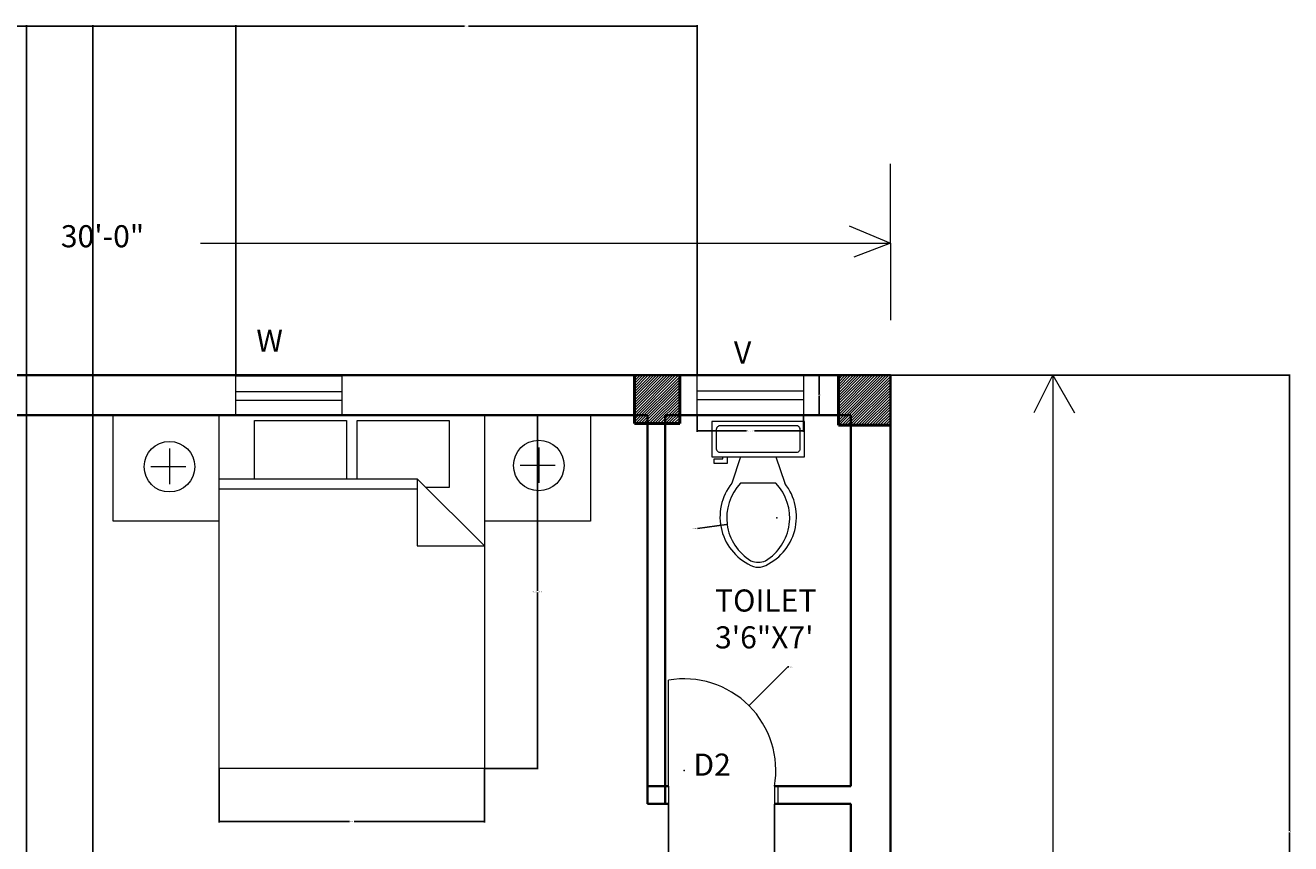
# Model space of a CAD drawing. Units: inches. Extents: x -12 to 472, y -585 to 99.
# Tile 4 of 4: x 186 to 472, y -86 to 99. Entities that reach past the tile are written whole.
import ezdxf

# ---------------------------------------------------------------- set-up
doc = ezdxf.new("R2010")
doc.units = ezdxf.units.IN
doc.header["$MEASUREMENT"] = 0
for name, color, linetype, lineweight in [('A-ANNO-DIMS', 2, 'Continuous', 18), ('A-ANNO-TEXT', 7, 'Continuous', 18), ('A-AREA-IDEN', 7, 'Continuous', 25), ('A-COLS', 7, 'Continuous', 50), ('A-COLS-PATT', 252, 'Continuous', 13), ('A-DOOR', 3, 'Continuous', 18), ('A-FLOR-FIXT', 9, 'Continuous', 20), ('A-FURN', 8, 'Continuous', 18), ('A-GLAZ', 4, 'Continuous', 18), ('A-WALL', 7, 'Continuous', 35)]:
    doc.layers.add(name, color=color, linetype=linetype, lineweight=lineweight)
doc.styles.get("Standard").update_dxf_attribs({"font": 'arial.ttf'})
doc.dimstyles.get("Standard").update_dxf_attribs({"dimtxt": 0.18, "dimasz": 0.18, "dimexe": 0.18, "dimexo": 0.0625, "dimgap": 0.09, "dimtad": 0, "dimtih": 1, "dimtoh": 1, "dimdec": 4, "dimzin": 0, "dimdsep": 46, "dimtxsty": 'Standard', "dimcen": 0.09, "dimadec": 0, "dimazin": 0, "dimtfac": 1, "dimtdec": 4, "dimtofl": 0, "dimtmove": 0, "dimatfit": 3, "dimfxl": 1, "dimtolj": 1, "dimtzin": 0, "dimarcsym": 0})
pattern_1 = [(45, (-1281.90016, -702.76037), (-0.30935922, 0.30935922), [])]

# ---------------------------------------------------------------- blocks, each defined once
blk = doc.blocks.new('Toilet - top')
for p, q in [((9.5, -6), (9.5, -2)), ((-10, -8.5), (-8, -8.5)), ((-10, -9.5), (-10, -8.5)), ((-8, -8.5), (-8, -8)), ((-7, -8), (-7, -9.5)), ((-4, -8), (-6, -14)), ((4, -8), (6, -14)), ((-7, -9.5), (-10, -9.5)), ((4, -14), (-4, -14))]:
    blk.add_line(p, q)
blk.add_lwpolyline([(10.5, -8), (10.5, 0), (-10.5, 0), (-10.5, -8)], close=True)
for points in [[(-9.5, -2), (-9.5, -6)], [(8.5, -1), (-8.5, -1)], [(-8.5, -7), (8.5, -7)]]:
    blk.add_lwpolyline(points)
for centre, radius, start, end in [((-8.62, -1.88), 0.884, 81.8699, 188.1301), ((8.62, -1.88), 0.884, 351.8699, 98.1301), ((-8.62, -6.12), 0.884, 171.8699, 278.1301), ((8.62, -6.12), 0.884, 261.8699, 8.1301), ((3.52, -21.58), 12.17, 141.4691, 247.9714), ((4.2, -21.82), 11.33, 136.3677, 238.9468), ((-3.52, -21.58), 12.17, 292.0284, 38.5307), ((-4.2, -21.82), 11.33, 301.053, 43.6321), ((0, -27.88), 4, 245.7318, 294.2682), ((0, -29), 4, 254.8605, 285.1395)]:
    blk.add_arc(centre, radius, start, end)
blk = doc.blocks.new('Bed - Queen')
for p, q in [((0, -80.00003), (0, 0)), ((0, 0), (59.99999, 0)), ((59.99999, 0), (59.99999, -80.00003)), ((7.99999, -1.2), (28.79998, -1.2)), ((7.99999, -14.4), (7.99999, -1.2)), ((28.79998, -1.2), (28.79998, -14.4)), ((31.19999, -1.2), (51.99999, -1.2)), ((31.19999, -14.4), (31.19999, -1.2)), ((51.99999, -1.2), (51.99999, -16.4)), ((0, -14.4), (44.8, -14.4)), ((44.8, -16.8), (0, -16.8)), ((59.99999, -29.6), (44.8, -14.4)), ((44.8, -14.4), (44.8, -29.6)), ((51.99999, -16.4), (46.79936, -16.4)), ((44.8, -29.6), (59.99999, -29.6)), ((59.99999, -80.00003), (0, -80.00003))]:
    blk.add_line(p, q)
blk = doc.blocks.new('WIN-24IN-EXT')
for p, q in [((0, 5.5), (24, 5.5)), ((0, 3.5), (24, 3.5))]:
    blk.add_line(p, q)
blk.add_lwpolyline([(0, 9), (24, 9), (24, 0), (0, 0)], close=True)
blk = doc.blocks.new('VENT-24IN-EXT')
for p, q in [((0, 5.5), (24, 5.5)), ((0, 3.5), (24, 3.5))]:
    blk.add_line(p, q)
blk.add_lwpolyline([(0, 9), (24, 9), (24, 0), (0, 0)], close=True)
blk = doc.blocks.new('NIGHTSTAND-24IN')
for p, q in [((0, 24), (24, 24)), ((24, 24), (24, 0)), ((24, 0), (0, 0))]:
    blk.add_line(p, q)
blk = doc.blocks.new('LAMP-BEDSIDE-PLAN')
for p, q in [((5.72, 9.81), (5.72, 1.79)), ((1.49, 5.8), (9.4, 5.8))]:
    blk.add_line(p, q)
blk.add_circle((5.72, 5.72), 5.72)
blk = doc.blocks.new('*D12')
at = {"layer": 'A-ANNO-DIMS', "color": 0, "lineweight": -2, "transparency": 16777216}
for p, q in [((337.57, 10.56), (337.57, 6.84)), ((361.57, 10.56), (361.57, 6.84)), ((337.75, 7.02), (348.67, 7.02)), ((361.39, 7.02), (350.48, 7.02))]:
    blk.add_line(p, q, dxfattribs=at)
at = {"layer": 'A-ANNO-DIMS', "color": 0, "transparency": 16777216}
for points in [[(337.75, 7.05), (337.75, 6.99), (337.57, 7.02)], [(361.39, 7.05), (361.39, 6.99), (361.57, 7.02)]]:
    blk.add_solid(points, dxfattribs=at)
at = {"layer": 'Defpoints', "color": 0, "transparency": 16777216}
for p in [(337.57, 10.62), (361.57, 10.62), (361.57, 7.02)]:
    blk.add_point(p, dxfattribs=at)
at = {"layer": 'A-ANNO-DIMS', "color": 0, "transparency": 16777216, "insert": (349.57, 7.02), "char_height": 0.18, "attachment_point": 5}
blk.add_mtext('\\A1;VENT 24 TYP.', dxfattribs=at)
blk = doc.blocks.new('*D13')
at = {"layer": 'A-ANNO-DIMS', "color": 0, "lineweight": -2, "transparency": 16777216}
for p, q in [((361.64, 19.62), (365.35, 19.62)), ((365.17, 19.44), (365.17, 15.3)), ((365.17, 10.8), (365.17, 14.94)), ((361.64, 10.62), (365.35, 10.62))]:
    blk.add_line(p, q, dxfattribs=at)
at = {"layer": 'A-ANNO-DIMS', "color": 0, "transparency": 16777216}
for points in [[(365.14, 19.44), (365.2, 19.44), (365.17, 19.62)], [(365.14, 10.8), (365.2, 10.8), (365.17, 10.62)]]:
    blk.add_solid(points, dxfattribs=at)
at = {"layer": 'Defpoints', "color": 0, "transparency": 16777216}
for p in [(361.57, 19.62), (365.17, 19.62), (361.57, 10.62)]:
    blk.add_point(p, dxfattribs=at)
at = {"layer": 'A-ANNO-DIMS', "color": 0, "transparency": 16777216, "insert": (365.17, 15.12), "char_height": 0.18, "attachment_point": 5}
blk.add_mtext('\\A1;9 TYP.', dxfattribs=at)
blk = doc.blocks.new('*D18')
at = {"layer": 'A-ANNO-DIMS', "color": 0, "lineweight": -2, "transparency": 16777216}
for p, q in [((289.49, 10.62), (301.61, 10.62)), ((301.43, 10.44), (301.43, -29.19)), ((301.43, -69.2), (301.43, -29.57)), ((289.49, -69.38), (301.61, -69.38))]:
    blk.add_line(p, q, dxfattribs=at)
at = {"layer": 'A-ANNO-DIMS', "color": 0, "transparency": 16777216}
for points in [[(301.4, 10.44), (301.46, 10.44), (301.43, 10.62)], [(301.4, -69.2), (301.46, -69.2), (301.43, -69.38)]]:
    blk.add_solid(points, dxfattribs=at)
at = {"layer": 'Defpoints', "color": 0, "transparency": 16777216}
for p in [(289.43, 10.62), (301.43, 10.62), (289.43, -69.38)]:
    blk.add_point(p, dxfattribs=at)
at = {"layer": 'A-ANNO-DIMS', "color": 0, "transparency": 16777216, "insert": (301.43, -29.38), "char_height": 0.18, "attachment_point": 5}
blk.add_mtext('\\A1;QUEEN BED 80 TYP.', dxfattribs=at)
blk = doc.blocks.new('*D19')
at = {"layer": 'A-ANNO-DIMS', "color": 0, "lineweight": -2, "transparency": 16777216}
for p, q in [((229.43, -69.44), (229.43, -81.56)), ((289.43, -69.44), (289.43, -81.56)), ((229.61, -81.38), (258.9, -81.38)), ((289.25, -81.38), (259.96, -81.38))]:
    blk.add_line(p, q, dxfattribs=at)
at = {"layer": 'A-ANNO-DIMS', "color": 0, "transparency": 16777216}
for points in [[(229.61, -81.35), (229.61, -81.41), (229.43, -81.38)], [(289.25, -81.35), (289.25, -81.41), (289.43, -81.38)]]:
    blk.add_solid(points, dxfattribs=at)
at = {"layer": 'Defpoints', "color": 0, "transparency": 16777216}
for p in [(229.43, -69.38), (289.43, -69.38), (289.43, -81.38)]:
    blk.add_point(p, dxfattribs=at)
at = {"layer": 'A-ANNO-DIMS', "color": 0, "transparency": 16777216, "insert": (259.43, -81.38), "char_height": 0.18, "attachment_point": 5}
blk.add_mtext('\\A1;60 TYP.', dxfattribs=at)
blk = doc.blocks.new('*D30')
at = {"layer": 'A-ANNO-DIMS', "color": 0, "lineweight": -2, "transparency": 16777216}
for p, q in [((185.8, -429.83), (185.8, 98.81)), ((185.98, 98.63), (193.09, 98.63)), ((200.62, 98.63), (193.51, 98.63)), ((200.8, -431.32), (200.8, 98.81))]:
    blk.add_line(p, q, dxfattribs=at)
at = {"layer": 'A-ANNO-DIMS', "color": 0, "transparency": 16777216}
for points in [[(185.98, 98.66), (185.98, 98.6), (185.8, 98.63)], [(200.62, 98.66), (200.62, 98.6), (200.8, 98.63)]]:
    blk.add_solid(points, dxfattribs=at)
at = {"layer": 'Defpoints', "color": 0, "transparency": 16777216}
for p in [(200.8, 98.63), (185.8, -429.9), (200.8, -431.38)]:
    blk.add_point(p, dxfattribs=at)
at = {"layer": 'A-ANNO-DIMS', "color": 0, "transparency": 16777216, "insert": (193.3, 98.63), "char_height": 0.18, "attachment_point": 5}
blk.add_mtext('\\A1;15', dxfattribs=at)
blk = doc.blocks.new('*D40')
at = {"layer": 'A-ANNO-DIMS', "color": 0, "lineweight": -2, "transparency": 16777216}
for p, q in [((331.04, -77.44), (331.04, -585.26)), ((355.04, -77.44), (355.04, -585.26)), ((331.22, -585.08), (342.82, -585.08)), ((354.86, -585.08), (343.26, -585.08))]:
    blk.add_line(p, q, dxfattribs=at)
at = {"layer": 'A-ANNO-DIMS', "color": 0, "transparency": 16777216}
for points in [[(331.22, -585.05), (331.22, -585.11), (331.04, -585.08)], [(354.86, -585.05), (354.86, -585.11), (355.04, -585.08)]]:
    blk.add_solid(points, dxfattribs=at)
at = {"layer": 'Defpoints', "color": 0, "transparency": 16777216}
for p in [(331.04, -77.38), (355.04, -77.38), (355.04, -585.08)]:
    blk.add_point(p, dxfattribs=at)
at = {"layer": 'A-ANNO-DIMS', "color": 0, "transparency": 16777216, "insert": (343.04, -585.08), "char_height": 0.18, "attachment_point": 5}
blk.add_mtext('\\A1;24', dxfattribs=at)
blk = doc.blocks.new('*D42')
at = {"layer": 'A-ANNO-DIMS', "color": 0, "lineweight": -2, "transparency": 16777216}
for p, q in [((74.01, 19.68), (74.01, 98.81)), ((74.19, 98.63), (153.13, 98.63)), ((232.97, 98.63), (154.04, 98.63)), ((233.15, 19.53), (233.15, 98.81))]:
    blk.add_line(p, q, dxfattribs=at)
at = {"layer": 'A-ANNO-DIMS', "color": 0, "transparency": 16777216}
for points in [[(74.19, 98.66), (74.19, 98.6), (74.01, 98.63)], [(232.97, 98.66), (232.97, 98.6), (233.15, 98.63)]]:
    blk.add_solid(points, dxfattribs=at)
at = {"layer": 'Defpoints', "color": 0, "transparency": 16777216}
for p in [(233.15, 98.63), (74.01, 19.62), (233.15, 19.47)]:
    blk.add_point(p, dxfattribs=at)
at = {"layer": 'A-ANNO-DIMS', "color": 0, "transparency": 16777216, "insert": (153.58, 98.63), "char_height": 0.18, "attachment_point": 5}
blk.add_mtext('\\A1;159.13', dxfattribs=at)
blk = doc.blocks.new('*D43')
at = {"layer": 'A-ANNO-DIMS', "color": 0, "lineweight": -2, "transparency": 16777216}
for p, q in [((233.15, 19.53), (233.15, 98.81)), ((233.33, 98.63), (284.91, 98.63)), ((337.39, 98.63), (285.81, 98.63)), ((337.57, 19.68), (337.57, 98.81))]:
    blk.add_line(p, q, dxfattribs=at)
at = {"layer": 'A-ANNO-DIMS', "color": 0, "transparency": 16777216}
for points in [[(233.33, 98.66), (233.33, 98.6), (233.15, 98.63)], [(337.39, 98.66), (337.39, 98.6), (337.57, 98.63)]]:
    blk.add_solid(points, dxfattribs=at)
at = {"layer": 'Defpoints', "color": 0, "transparency": 16777216}
for p in [(337.57, 98.63), (233.15, 19.47), (337.57, 19.62)]:
    blk.add_point(p, dxfattribs=at)
at = {"layer": 'A-ANNO-DIMS', "color": 0, "transparency": 16777216, "insert": (285.36, 98.63), "char_height": 0.18, "attachment_point": 5}
blk.add_mtext('\\A1;104.42', dxfattribs=at)
blk = doc.blocks.new('*D50')
at = {"layer": 'A-ANNO-DIMS', "color": 0, "lineweight": -2, "transparency": 16777216}
for p, q in [((381.34, 19.62), (471.69, 19.62)), ((471.51, 19.44), (471.51, -83.45)), ((471.51, -186.7), (471.51, -83.81)), ((381.34, -186.88), (471.69, -186.88))]:
    blk.add_line(p, q, dxfattribs=at)
at = {"layer": 'A-ANNO-DIMS', "color": 0, "transparency": 16777216}
for points in [[(471.48, 19.44), (471.54, 19.44), (471.51, 19.62)], [(471.48, -186.7), (471.54, -186.7), (471.51, -186.88)]]:
    blk.add_solid(points, dxfattribs=at)
at = {"layer": 'Defpoints', "color": 0, "transparency": 16777216}
for p in [(381.28, 19.62), (381.28, -186.88), (471.51, -186.88)]:
    blk.add_point(p, dxfattribs=at)
at = {"layer": 'A-ANNO-DIMS', "color": 0, "transparency": 16777216, "insert": (471.51, -83.63), "char_height": 0.18, "attachment_point": 5}
blk.add_mtext('\\A1;206.5', dxfattribs=at)
blk = doc.blocks.new('*D59')
at = {"layer": 'A-ANNO-DIMS', "color": 0, "lineweight": -2, "transparency": 16777216}
for p, q in [((358.07, -46.35), (349.4, -55.02)), ((358.25, -46.35), (358.07, -46.35)), ((334.51, -69.82), (334.69, -69.82)), ((334.6, -69.91), (334.6, -69.73))]:
    blk.add_line(p, q, dxfattribs=at)
at = {"layer": 'A-ANNO-DIMS', "color": 0, "transparency": 16777216}
blk.add_solid([(349.38, -55), (349.42, -55.04), (349.27, -55.15)], dxfattribs=at)
at = {"layer": 'Defpoints', "color": 0, "transparency": 16777216}
for p in [(349.27, -55.15), (334.6, -69.82)]:
    blk.add_point(p, dxfattribs=at)
at = {"layer": 'A-ANNO-DIMS', "color": 0, "transparency": 16777216, "insert": (358.81, -46.35), "char_height": 0.18, "attachment_point": 5}
blk.add_mtext('\\A1;R20.745', dxfattribs=at)
blk = doc.blocks.new('*D63')
at = {"layer": 'A-ANNO-DIMS', "color": 0, "lineweight": -2, "transparency": 16777216}
for p, q in [((337.59, -15.05), (344.15, -14.17)), ((355.47, -12.63), (355.65, -12.63)), ((355.56, -12.72), (355.56, -12.54))]:
    blk.add_line(p, q, dxfattribs=at)
at = {"layer": 'A-ANNO-DIMS', "color": 0, "transparency": 16777216}
blk.add_solid([(344.15, -14.14), (344.16, -14.2), (344.33, -14.15)], dxfattribs=at)
at = {"layer": 'Defpoints', "color": 0, "transparency": 16777216}
for p in [(344.33, -14.15), (355.56, -12.63)]:
    blk.add_point(p, dxfattribs=at)
at = {"layer": 'A-ANNO-DIMS', "color": 0, "transparency": 16777216, "insert": (336.92, -15.05), "char_height": 0.18, "attachment_point": 5}
blk.add_mtext('\\A1;4X R11.33', dxfattribs=at)

msp = doc.modelspace()

# ---------------------------------------------------------------- hatches: boundary and pattern name
at = {"layer": 'A-COLS-PATT'}
h = msp.add_hatch(dxfattribs=at)
h.set_pattern_fill('ANSI31', color=256, scale=3.5)
h.set_pattern_definition(pattern_1)
h.paths.add_polyline_path([(333.5896, 19.6212), (323.3586, 19.6212), (323.3586, 10.6212), (326.2783, 10.6212), (326.2783, 8.6749), (330.2783, 8.6749), (330.2783, 10.6212), (333.5896, 10.6212)])
h.paths.add_polyline_path([(326.2783, 10.6212), (323.3586, 10.6212), (323.3586, 8.6749), (326.2783, 8.6749)], flags=17)
h.paths.add_polyline_path([(333.5896, 10.6212), (330.2783, 10.6212), (330.2783, 8.6749), (333.5896, 8.6749)], flags=17)
h = msp.add_hatch(dxfattribs=at)
h.set_pattern_fill('ANSI31', color=256, scale=3.5)
h.set_pattern_definition(pattern_1)
h.paths.add_polyline_path([(381.2783, 19.6212), (369.4843, 19.6212), (369.4843, 10.6212), (372.2783, 10.6212), (372.2783, 8.3052), (381.2783, 8.3052)])
h.paths.add_polyline_path([(372.2783, 10.6212), (369.4843, 10.6212), (369.4843, 8.3052), (372.2783, 8.3052)], flags=17)

# ---------------------------------------------------------------- linework, layer by layer
at = {"layer": 'A-ANNO-DIMS'}
for p, q in [((381.2783, 49.4723), (381.2783, 67.4273)), ((371.9373, 53.4061), (381.2783, 49.4723)), ((225.2164, 49.4723), (381.2783, 49.4723)), ((381.2783, 49.4723), (373.0078, 46.3222)), ((381.2783, 49.4723), (381.2783, 32.0533)), ((395.6851, 19.6212), (440.3096, 19.6212)), ((413.8214, 11.17), (417.9974, 19.6212)), ((417.9974, 19.6212), (417.9974, -233.6801)), ((417.9974, 19.6212), (422.9031, 11.1243))]:
    msp.add_line(p, q, dxfattribs=at)
at = {"layer": 'A-COLS'}
for p, q in [((323.3586, 19.6212), (323.3586, 8.6749)), ((333.5896, 8.6749), (333.5896, 19.6212)), ((369.4843, 19.6212), (369.4843, 8.3052)), ((323.3586, 8.6749), (333.5896, 8.6749)), ((369.4843, 8.3052), (381.2783, 8.3052))]:
    msp.add_line(p, q, dxfattribs=at)
at = {"layer": 'A-DOOR'}
for p, q in [((331.0411, -73.3788), (331.0411, -49.3788)), ((331.0411, -73.3788), (331.0411, -77.3788)), ((355.0411, -73.3788), (355.0411, -77.3788)), ((355.8166, -73.3788), (355.8166, -77.3788))]:
    msp.add_line(p, q, dxfattribs=at)
msp.add_arc((334.6042, -69.8156), 20.7452, 350.10998, 99.89002, dxfattribs=at)
at = {"layer": 'A-WALL'}
for p, q in [((178.2783, 10.6212), (326.2783, 10.6212)), ((326.2783, 10.6212), (326.2783, -77.3788)), ((330.2783, 10.6212), (330.2783, -77.3788)), ((330.2783, 10.6212), (372.2783, 10.6212)), ((372.2783, 10.6212), (372.2783, -73.3788)), ((326.2783, -73.3788), (331.0411, -73.3788)), ((355.0411, -73.3788), (372.2783, -73.3788)), ((326.2783, -77.3788), (331.0411, -77.3788)), ((355.0411, -77.3788), (372.2783, -77.3788)), ((372.2783, -77.3788), (372.2783, -133.3788))]:
    msp.add_line(p, q, dxfattribs=at)
msp.add_lwpolyline([(21.2783, 19.6212), (381.2783, 19.6212), (381.2783, -526.3788), (21.2783, -526.3788)], close=True, dxfattribs=at)

# ---------------------------------------------------------------- block references
at = {"layer": 'A-FLOR-FIXT'}
msp.add_blockref('Toilet - top', (351.3581, 9.1824), dxfattribs=at)
at = {"layer": 'A-FURN', "rotation": 180}
msp.add_blockref('NIGHTSTAND-24IN', (229.428, 10.6214), dxfattribs=at)
at = {"layer": 'A-FURN'}
for name, p in [('Bed - Queen', (229.428, 10.6212)), ('NIGHTSTAND-24IN', (289.428, -13.3789)), ('LAMP-BEDSIDE-PLAN', (212.4458, -6.7945)), ('LAMP-BEDSIDE-PLAN', (295.9994, -6.5204))]:
    msp.add_blockref(name, p, dxfattribs=at)
at = {"layer": 'A-GLAZ'}
for name, p in [('WIN-24IN-EXT', (233.1479, 10.4678)), ('VENT-24IN-EXT', (337.573, 10.621))]:
    msp.add_blockref(name, p, dxfattribs=at)

# ---------------------------------------------------------------- texts
at = {"layer": 'A-ANNO-DIMS', "insert": (193.5858, 53.578), "char_height": 5, "attachment_point": 1}
msp.add_mtext_dynamic_manual_height_columns('30\'-0"', width=25.438653, gutter_width=25, heights=[0], dxfattribs=at)
at = {"layer": 'A-ANNO-TEXT', "char_height": 5, "attachment_point": 1}
for s, width, insert in [('W', 11.331186, (237.8264, 29.9341)), ('V', 17.014562, (345.8614, 27.2685)), ('D2', 15.456514, (336.686, -65.9853))]:
    msp.add_mtext_dynamic_manual_height_columns(s, width=width, gutter_width=25, heights=[0], dxfattribs=dict(at, insert=insert))
at = {"layer": 'A-AREA-IDEN', "insert": (341.5854, -28.8525), "char_height": 5, "attachment_point": 1}
msp.add_mtext_dynamic_manual_height_columns('TOILET\\P3\'6"X7\'', width=38.514755, gutter_width=25, heights=[0], dxfattribs=at)

# ---------------------------------------------------------------- dimensions: what is measured, and where the dimension line sits
at = {"layer": 'A-ANNO-DIMS'}
for base, p1, p2, override, picture, middle in [((233.1482, 98.6273), (74.0143, 19.6212), (233.1482, 19.468), {"dimdec": 2, "dimlfac": 1, "dimrnd": 0, "dimzin": 0, "dimdsep": 46, "dimlunit": 2}, '*D42', (153.5813, 98.6273)), ((200.803, 98.6273), (185.8034, -429.897), (200.803, -431.3788), {"dimdec": 0, "dimlfac": 1, "dimrnd": 0, "dimzin": 0, "dimdsep": 46, "dimlunit": 2}, '*D30', (193.3032, 98.6273)), ((337.5728, 98.6273), (233.1482, 19.468), (337.5728, 19.6212), {"dimdec": 2, "dimlfac": 1, "dimrnd": 0, "dimzin": 0, "dimdsep": 46, "dimlunit": 2}, '*D43', (285.3605, 98.6273)), ((355.0411, -585.0813), (331.0411, -77.3788), (355.0411, -77.3788), {"dimdec": 0, "dimlfac": 1, "dimrnd": 0, "dimzin": 0, "dimdsep": 46, "dimlunit": 2}, '*D40', (343.0411, -585.0813))]:
    dim = msp.add_linear_dim(base=base, p1=p1, p2=p2, dimstyle='Standard', override=override, dxfattribs=at)
    dim.commit()
    dim.dimension.update_dxf_attribs({"geometry": picture, "text_midpoint": middle})
for base, p1, p2, text, picture, middle in [((365.1728, 19.6212), (361.5728, 10.6212), (361.5728, 19.6212), '<> TYP.', '*D13', (365.1728, 15.1212)), ((301.428, 10.6212), (289.428, -69.3788), (289.428, 10.6212), 'QUEEN BED <> TYP.', '*D18', (301.428, -29.3788))]:
    dim = msp.add_linear_dim(base=base, p1=p1, p2=p2, angle=90, text=text, dimstyle='Standard', override={"dimdec": 0, "dimlfac": 1, "dimrnd": 0, "dimzin": 0, "dimdsep": 46, "dimlunit": 2}, dxfattribs=at)
    dim.commit()
    dim.dimension.update_dxf_attribs({"geometry": picture, "text_midpoint": middle})
dim = msp.add_linear_dim(base=(471.5096, -186.8788), p1=(381.2783, 19.6212), p2=(381.2783, -186.8788), angle=90, dimstyle='Standard', override={"dimdec": 1, "dimlfac": 1, "dimrnd": 0, "dimzin": 0, "dimdsep": 46, "dimlunit": 2}, dxfattribs=at)
dim.commit()
dim.dimension.update_dxf_attribs({"geometry": '*D50', "text_midpoint": (471.5096, -83.6288)})
for base, p1, p2, text, picture, middle in [((361.5728, 7.0212), (337.5728, 10.6212), (361.5728, 10.6212), 'VENT <> TYP.', '*D12', (349.5728, 7.0212)), ((289.428, -81.3788), (229.428, -69.3788), (289.428, -69.3788), '<> TYP.', '*D19', (259.428, -81.3788))]:
    dim = msp.add_linear_dim(base=base, p1=p1, p2=p2, text=text, dimstyle='Standard', override={"dimdec": 0, "dimlfac": 1, "dimrnd": 0, "dimzin": 0, "dimdsep": 46, "dimlunit": 2}, dxfattribs=at)
    dim.commit()
    dim.dimension.update_dxf_attribs({"geometry": picture, "text_midpoint": middle})
dim = msp.add_radius_dim(center=(355.558, -12.635), mpoint=(344.3299, -14.145), text='4X <>', dimstyle='Standard', override={"dimdec": 2, "dimlfac": 1, "dimrnd": 0, "dimzin": 0, "dimdsep": 46, "dimlunit": 2}, dxfattribs=at)
dim.commit()
dim.dimension.update_dxf_attribs({"geometry": '*D63', "text_midpoint": (337.5931, -15.051), "dimtype": 164})
dim = msp.add_radius_dim(center=(334.6042, -69.8156), mpoint=(349.2733, -55.1467), dimstyle='Standard', override={"dimdec": 3, "dimlfac": 1, "dimrnd": 0, "dimzin": 0, "dimdsep": 46, "dimlunit": 2}, dxfattribs=at)
dim.commit()
dim.dimension.update_dxf_attribs({"geometry": '*D59', "text_midpoint": (358.8052, -46.3453), "dimtype": 164})

doc.saveas('drawing.dxf')
